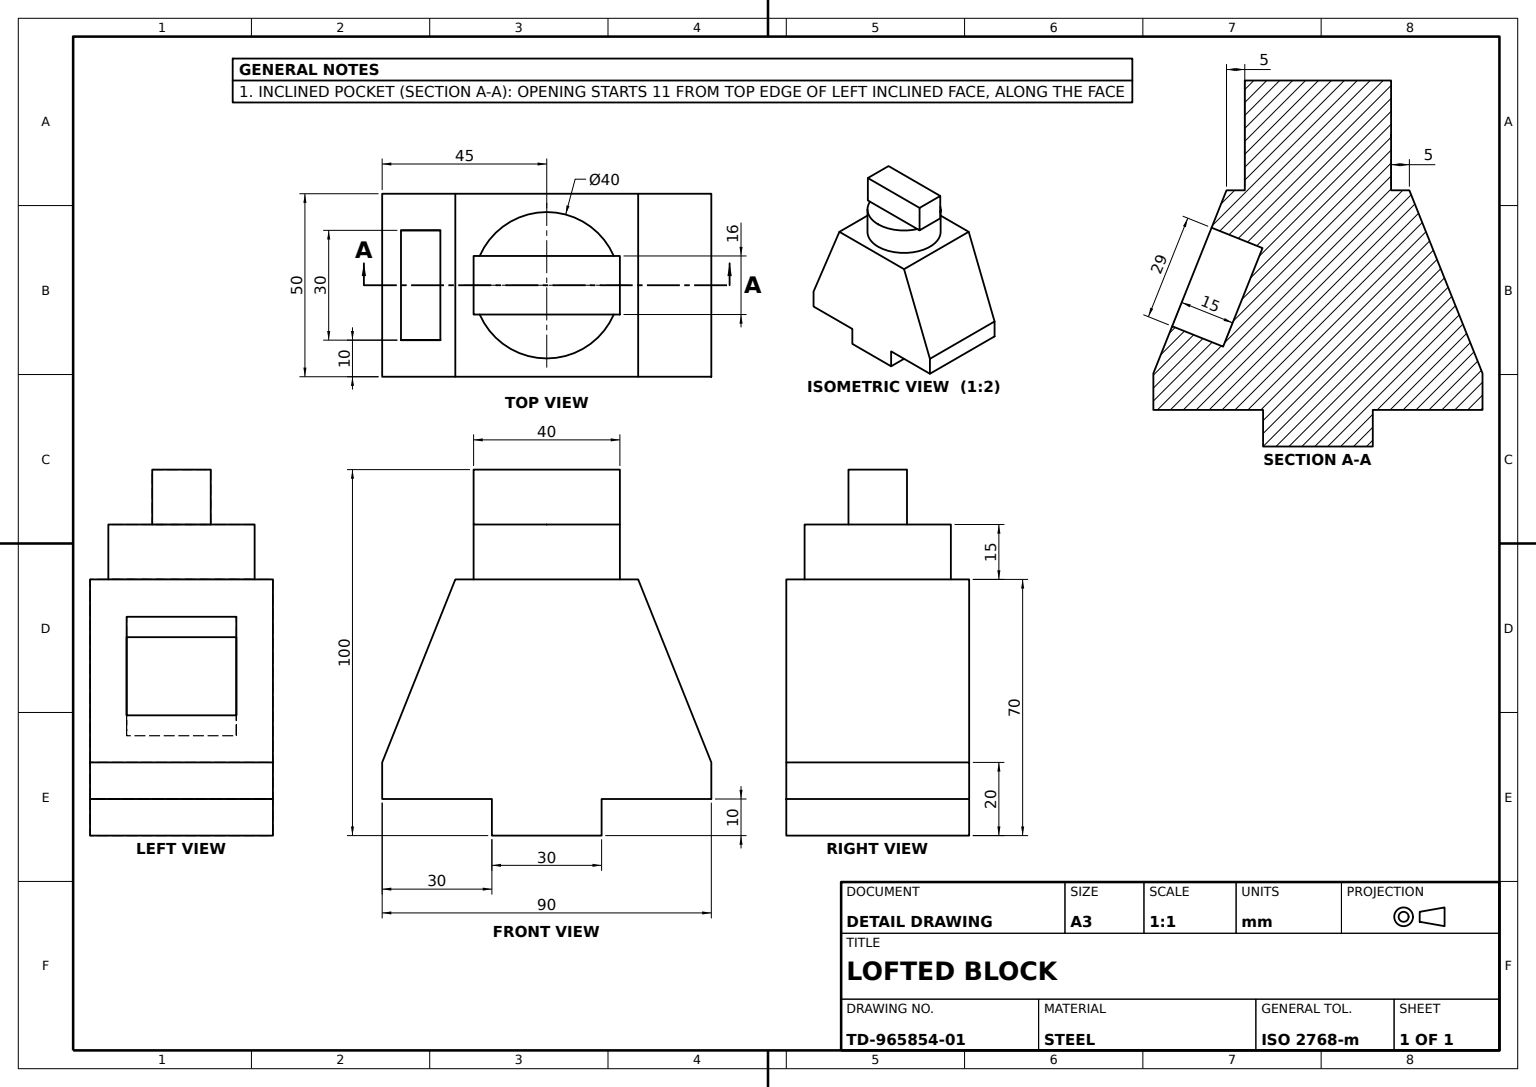
SolidWorks part; units mm, degrees
material "Plain Carbon Steel"
ref_plane "Front Plane" through (0, 0, 0) normal (0, 0, 1) x (1, 0, 0)
ref_plane "Top Plane" through (0, 0, 0) normal (0, 1, 0) x (1, 0, 0)
ref_plane "Right Plane" through (0, 0, 0) normal (1, 0, 0) x (0, 0, -1)
sketch "Base Profile Sketch" plane through (0, 0, 0) normal (0, 0, 1) x (1, 0, 0)
  line L0 (15, -5) -> (45, -5)
  line L1 (-45, 5) -> (45, 5)
  line L2 (-45, 5) -> (-45, -5)
  line L3 (-45, -5) -> (-15, -5)
  line L4 (45, 5) -> (45, -5)
  line L8 (-15, -5) -> (-15, -15)
  line L9 (-15, -15) -> (15, -15)
  line L10 (15, -5) -> (15, -15)
  point P0 (0, 0)
  point P6 (0, -5)
  dimension "D1" = 10
  dimension "D2" = 90
  dimension "D3" = 10
  dimension "D4" = 30
  dimension "D5" = 30
  dimension "D6" = 5
  dimension "D7" = 45
extrude "Base Block" add sketch "Base Profile Sketch" along normal blind 50
ref_plane "Loft Top Plane" through (0, 55, 0) normal (0, 1, 0) x (1, 0, 0)
sketch "Loft Top Profile Sketch" plane through (0, 55, 0) normal (0, 1, 0) x (1, 0, 0)
  line L0 (45, 0) -> (-45, 0) construction
  line L1 (-25, 0) -> (25, 0)
  line L2 (-25, 0) -> (-25, -50)
  line L3 (-25, -50) -> (25, -50)
  line L4 (25, 0) -> (25, -50)
  line L5 (-25, 0) -> (25, -50) construction
  line L6 (-25, -50) -> (25, 0) construction
  line L7 (45, -50) -> (-45, -50) construction
  point P0 (0, -25)
  dimension "D1" = 50
loft "Tapered Body Loft" add profiles "Loft Top Profile Sketch" section "Loft Top Profile Sketch" section face at (0, 5, 25)
sketch "Round Boss Sketch" plane through (0, 55, 0) normal (0, 1, 0) x (1, 0, 0)
  line L0 (25, 0) -> (-25, 0) construction
  circle A0 centre (0, -25) radius 20
  dimension "D1" = 40
  dimension "D2" = 25
extrude "Round Boss" add sketch "Round Boss Sketch" along normal blind 15
sketch "Top Key Sketch" plane through (0, 70, 0) normal (0, 1, 0) x (1, 0, 0)
  line L1 (-20, -17) -> (20, -17)
  line L2 (-20, -17) -> (-20, -33)
  line L3 (-20, -33) -> (20, -33)
  line L4 (20, -17) -> (20, -33)
  line L5 (-20, -17) -> (20, -33) construction
  line L6 (-20, -33) -> (20, -17) construction
  point P0 (0, -25)
  dimension "D1" = 16
  dimension "D2" = 40
extrude "Top Key" add sketch "Top Key Sketch" along normal blind 15
sketch "Slot Sketch" plane through (-40.5172, 16.2069, 0) normal (-0.9285, 0.3714, 0) x (0, 0, 1)
  line L0 (0, 41.7815) -> (50, 41.7815) construction
  line L1 (10, 30.7815) -> (40, 30.7815)
  line L2 (10, 30.7815) -> (10, 1.7815)
  line L3 (10, 1.7815) -> (40, 1.7815)
  line L4 (40, 30.7815) -> (40, 1.7815)
  line L5 (10, 30.7815) -> (40, 1.7815) construction
  line L6 (10, 1.7815) -> (40, 30.7815) construction
  line L11 (50, 41.7815) -> (50, -12.0702) construction
  point P0 (25, 16.2815)
  dimension "D1" = 30
  dimension "D2" = 29
  dimension "D3" = 11
  dimension "D4" = 10
extrude "Slot Cut" cut sketch "Slot Sketch" against normal blind 15
